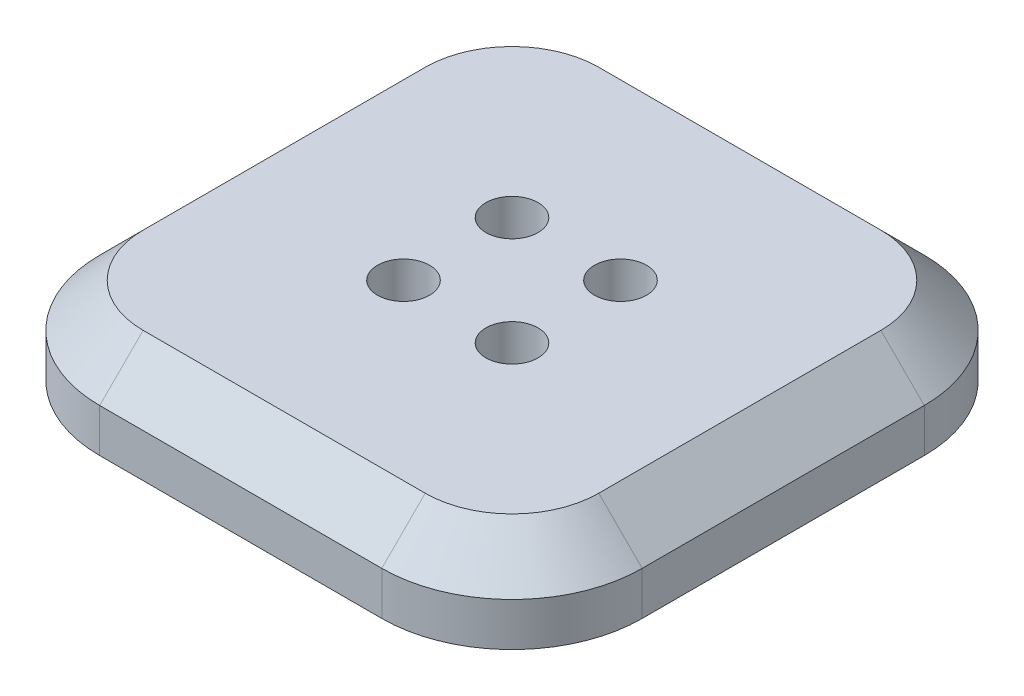
SolidWorks part; units mm, degrees
material "Plain Carbon Steel"
ref_plane "Front Plane" through (0, 0, 0) normal (0, 0, 1) x (1, 0, 0)
ref_plane "Top Plane" through (0, 0, 0) normal (0, 1, 0) x (1, 0, 0)
ref_plane "Right Plane" through (0, 0, 0) normal (1, 0, 0) x (0, 0, -1)
sketch "Base Plate Profile 125x125" plane through (0, 0, 0) normal (0, 1, 0) x (1, 0, 0)
  line L1 (-62.5, -62.5) -> (62.5, -62.5)
  line L2 (-62.5, -62.5) -> (-62.5, 62.5)
  line L3 (-62.5, 62.5) -> (62.5, 62.5)
  line L4 (62.5, -62.5) -> (62.5, 62.5)
  line L5 (-62.5, -62.5) -> (62.5, 62.5) construction
  line L6 (-62.5, 62.5) -> (62.5, -62.5) construction
  point P0 (0, 0)
  dimension "D1" = 125
  dimension "D2" = 125
extrude "Base Plate 20mm" add sketch "Base Plate Profile 125x125" along normal blind 20
fillet "Corner Fillets R30" radius 30 4 edges at (-62.5, 10, -62.5) (62.5, 10, -62.5) (62.5, 10, 62.5) (-62.5, 10, 62.5)
chamfer "Edge Chamfer 10x45°" distance 10 angle 45 8 edges at (-62.5, 20, 0) (-53.7132, 20, 53.7132) (-53.7132, 20, -53.7132) (0, 20, 62.5) (0, 20, -62.5) (53.7132, 20, 53.7132) (53.7132, 20, -53.7132) (62.5, 20, 0)
sketch "Dowel Hole Positions A" plane through (0, 20, 0) normal (0, 1, 0) x (1, 0, 0)
  line L1 (-12.5, -12.5) -> (12.5, -12.5)
  line L2 (-12.5, -12.5) -> (-12.5, 12.5)
  line L3 (-12.5, 12.5) -> (12.5, 12.5)
  line L4 (12.5, -12.5) -> (12.5, 12.5)
  line L5 (-12.5, -12.5) -> (12.5, 12.5) construction
  line L6 (-12.5, 12.5) -> (12.5, -12.5) construction
  point P0 (0, 0)
  dimension "D1" = 25
  dimension "D2" = 25
hole_wizard "Dowel Holes Ø12x10 A" positions "3DSketch1" profile "Sketch3" hole size "Ø12.0" standard "ANSI Metric"
sketch3d "3DSketch1"
  point P0 (-12.5, 20, -12.5)
  point P3 (12.5, 20, -12.5)
  point P6 (12.5, 20, 12.5)
  point P9 (-12.5, 20, 12.5)
sketch "Sketch3" plane through (-12.5, 20, -12.5) normal (1, 0, 0) x (0, 0, 1)
  line L0 (0, 0) -> (0, 13.6052)
  line L1 (0, 13.6052) -> (6, 10)
  line L2 (6, 10) -> (6, 0)
  line L5 (6, 0) -> (0, 0)
  line L10 (0, 13.6052) -> (-6, 10) construction
  line L11 (0, -6.35) -> (0, 107.95) construction
  dimension "Hole Dia." = 12
  dimension "Hole Depth" = 10
  dimension "Drill Angle" = 118
sketch "Dowel Hole Positions B" plane through (0, 0, 0) normal (0, -1, 0) x (1, 0, 0)
  line L1 (-37.5, -37.5) -> (37.5, -37.5)
  line L2 (-37.5, -37.5) -> (-37.5, 37.5)
  line L3 (-37.5, 37.5) -> (37.5, 37.5)
  line L4 (37.5, -37.5) -> (37.5, 37.5)
  line L5 (-37.5, -37.5) -> (37.5, 37.5) construction
  line L6 (-37.5, 37.5) -> (37.5, -37.5) construction
  point P0 (0, 0)
  dimension "D1" = 75
  dimension "D2" = 75
hole_wizard "Dowel Holes Ø12x10 B" positions "3DSketch2" profile "Sketch5" hole size "Ø12.0" standard "ANSI Metric"
sketch3d "3DSketch2"
  point P0 (-37.5, 0, 37.5)
  point P3 (37.5, 0, 37.5)
  point P6 (37.5, 0, -37.5)
  point P9 (-37.5, 0, -37.5)
sketch "Sketch5" plane through (-37.5, 0, 37.5) normal (1, 0, 0) x (0, 0, -1)
  line L0 (0, 0) -> (0, 13.6052)
  line L1 (0, 13.6052) -> (6, 10)
  line L2 (6, 10) -> (6, 0)
  line L5 (6, 0) -> (0, 0)
  line L10 (0, 13.6052) -> (-6, 10) construction
  line L11 (0, -6.35) -> (0, 107.95) construction
  dimension "Hole Dia." = 12
  dimension "Hole Depth" = 10
  dimension "Drill Angle" = 118
